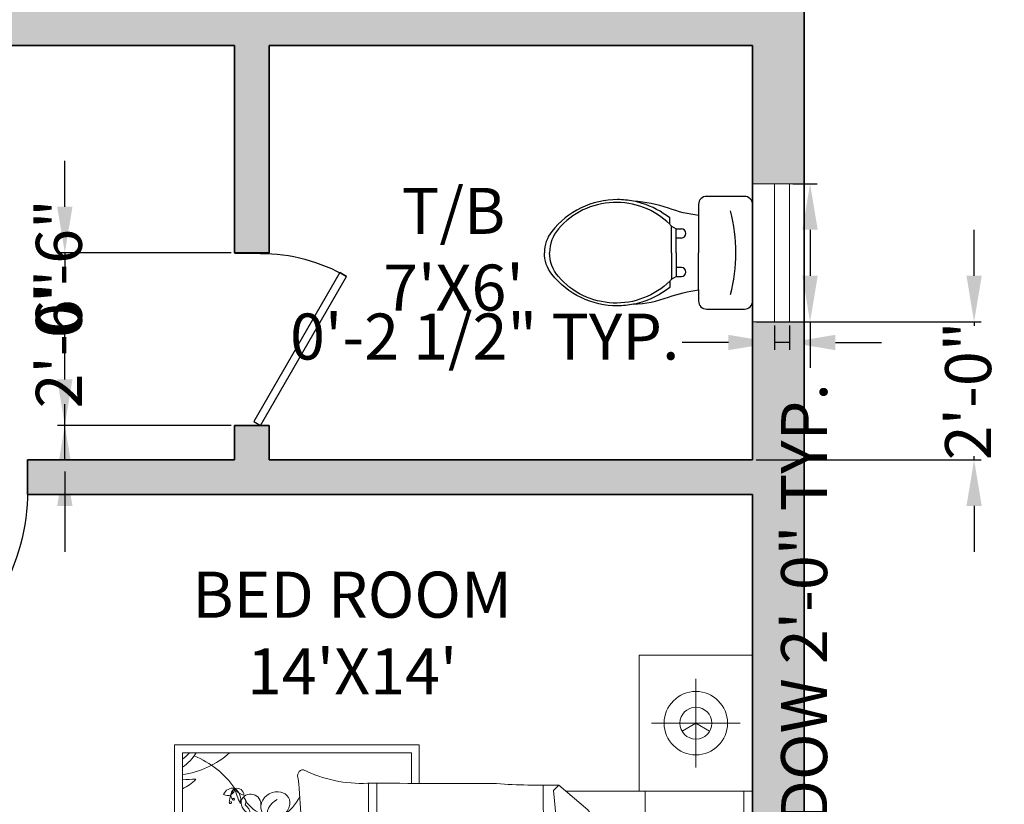
# Model space of a CAD drawing. Units: inches. Extents: x 2073 to 2646, y 2372 to 3017.
# Tile 3 of 8: x 2396 to 2567, y 2550 to 2686. Entities that reach past the tile are written whole.
import ezdxf

# ---------------------------------------------------------------- set-up
doc = ezdxf.new("R2010")
doc.units = ezdxf.units.IN
for name, color, linetype, lineweight in [('A-ANNO-DIMS', 2, 'Continuous', 18), ('A-AREA-IDEN', 7, 'Continuous', 25), ('A-DOOR', 3, 'Continuous', 25), ('A-FLOR-FIXT', 9, 'Continuous', 18), ('A-FURN', 8, 'Continuous', 18), ('A-GLAZ', 4, 'Continuous', 18), ('A-WALL', 7, 'Continuous', 35), ('A-WALL-PATT', 30, 'Continuous', 13)]:
    doc.layers.add(name, color=color, linetype=linetype, lineweight=lineweight)
doc.layers.add('WC-Detail_dwgmodels.com', color=251, linetype='Continuous')
doc.layers.add('WC-Outline_dwgmodels.com', color=250, linetype='Continuous')
doc.styles.get("Standard").update_dxf_attribs({"font": 'arial.ttf'})
doc.dimstyles.new('ISO-25', dxfattribs={"dimtxt": 8, "dimasz": 8, "dimexe": 1.25, "dimexo": 0.625, "dimtad": 0, "dimdec": 1, "dimlunit": 4, "dimtxsty": 'Standard', "dimcen": 2.5, "dimadec": 0, "dimazin": 0, "dimtfac": 1, "dimtdec": 1, "dimtmove": 0, "dimatfit": 3, "dimfxl": 1, "dimarcsym": 0})

# ---------------------------------------------------------------- blocks, each defined once
blk = doc.blocks.new('pan')
at = {"layer": 'WC-Detail_dwgmodels.com'}
for p, q in [((2373.44, 3021.91), (2373.44, 3022.64)), ((2374.73, 3022.64), (2374.73, 3021.91)), ((2378.86, 3022.64), (2378.86, 3021.91)), ((2380.15, 3021.91), (2380.15, 3022.64)), ((2373.08, 3021.25), (2373.44, 3021.91)), ((2374.73, 3021.91), (2373.44, 3021.91)), ((2376.79, 3021.91), (2374.73, 3021.91)), ((2376.79, 3021.91), (2378.86, 3021.91)), ((2378.86, 3021.91), (2380.15, 3021.91)), ((2380.51, 3021.25), (2380.15, 3021.91))]:
    blk.add_line(p, q, dxfattribs=at)
for points in [[(2373.08, 3021.25, 0.008985), (2372.8, 3020.99, 0.182634)], [(2376.79, 3021.25), (2373.08, 3021.25, 0.008985)], [(2376.79, 3021.25), (2380.51, 3021.25, -0.444938)], [(2380.51, 3021.25, -0.008985), (2380.79, 3020.99, -0.182634)], [(2372.8, 3020.99, 0.434217), (2373.44, 3005.35, 0.182634), (2376.79, 3004.12, 2.693815)], [(2371.91, 3020.99, 0.094048), (2369.85, 3017.12, 0.16845)], [(2372.8, 3020.99), (2371.91, 3020.99, 0.416606)], [(2380.79, 3020.99, -0.434217), (2380.15, 3005.35, -0.182634), (2376.79, 3004.12, -2.693815)], [(2380.79, 3020.99), (2381.68, 3020.99, -0.416606)], [(2381.68, 3020.99, -0.105447), (2383.88, 3016.61, -0.16845)], [(2369.85, 3017.12, 0.026594), (2369.55, 3015.91, 0.16845)], [(2383.88, 3016.61, -0.015301), (2384.04, 3015.91, -0.16845)]]:
    blk.add_lwpolyline(points, format="xyb", dxfattribs=at)
for centre, radius, start, end in [((2376.81, 3007.03), 23.26, 90.028, 104.6712), ((2376.78, 3007.03), 23.26, 75.3288, 89.972), ((2374.08, 3022.64), 0.645, 0, 180), ((2379.51, 3022.64), 0.645, 0, 180)]:
    blk.add_arc(centre, radius, start, end, dxfattribs=at)
at = {"layer": 'WC-Outline_dwgmodels.com'}
for points in [[(2383.59, 3025.06, 0.414214), (2384.72, 3026.19), (2384.72, 3031.5, 0.414214), (2383.59, 3032.64), (2376.79, 3032.64), (2370, 3032.64, 0.414214), (2368.87, 3031.5), (2368.87, 3026.19, 0.414214), (2370, 3025.06), (2371.56, 3025.06, -0.052345), (2370.54, 3020.81, 0.071131), (2369.55, 3015.91, 0.160777)], [(2371.56, 3025.06), (2376.79, 3025.06, 0.414214)], [(2382.03, 3025.06), (2376.79, 3025.06, -0.414214)], [(2384.04, 3015.91, 0.071131), (2383.05, 3020.81, -0.052345), (2382.03, 3025.06), (2383.59, 3025.06, 0.414214)], [(2369.55, 3015.91, 0.048023), (2369.32, 3013.67, 0.16845)], [(2384.04, 3015.91, -0.048023), (2384.27, 3013.67, -0.16845)], [(2369.32, 3013.67, 0.230343), (2373.8, 3004.42, 0.16845), (2376.79, 3003.38, 2.883082)], [(2384.27, 3013.67, -0.230343), (2379.79, 3004.42, -0.16845), (2376.79, 3003.38, -2.883082)]]:
    blk.add_lwpolyline(points, format="xyb", dxfattribs=at)
blk = doc.blocks.new('bed')
at = {"color": 0}
for p, q in [((2249.53, 3172.75), (2367.64, 3172.75)), ((2273.15, 3172.75), (2273.15, 3140.33)), ((2261.34, 3155.19), (2261.34, 3170.62)), ((2344.02, 3171.23), (2273.15, 3171.23)), ((2355.83, 3155.19), (2355.83, 3170.62)), ((2269.06, 3162.9), (2253.62, 3162.9)), ((2348.11, 3162.9), (2363.55, 3162.9)), ((2273.15, 3154.08), (2344.02, 3154.08)), ((2289.56, 3150.57), (2302.44, 3154.08)), ((2305.6, 3154.08), (2299.13, 3145.07)), ((2280.95, 3147.46), (2289.56, 3150.57)), ((2343.7, 3149.18), (2301.65, 3148.59)), ((2276.4, 3144.12), (2280.95, 3147.46)), ((2343.66, 3147.96), (2300.77, 3147.36)), ((2299.13, 3145.07), (2296.5, 3138.14)), ((2272.09, 3139.1), (2276.4, 3144.12)), ((2343.6, 3143.03), (2298.28, 3142.85)), ((2343.59, 3144.24), (2298.75, 3144.07)), ((2273.05, 3138.14), (2272.09, 3139.1)), ((2277.84, 3138.62), (2273.05, 3138.14)), ((2283.82, 3138.14), (2277.84, 3138.62)), ((2289.08, 3137.42), (2283.82, 3138.14)), ((2296.5, 3138.14), (2296.02, 3135.03)), ((2292.19, 3135.99), (2289.08, 3137.42)), ((2296.02, 3135.03), (2292.19, 3135.99)), ((2265.12, 3114.85), (2271.8, 3114.85)), ((2265.12, 3072.3), (2265.12, 3114.85)), ((2344.68, 3114.85), (2351.23, 3114.85)), ((2351.23, 3114.85), (2351.23, 3072.3)), ((2271.8, 3113.48), (2266.49, 3113.48)), ((2266.49, 3113.48), (2266.49, 3073.67)), ((2349.86, 3113.48), (2344.65, 3113.48)), ((2349.86, 3073.67), (2349.86, 3113.48)), ((2344.56, 3107.48), (2271.79, 3107.48)), ((2344.67, 3106.01), (2271.79, 3106.01)), ((2332.56, 3094.41), (2284.61, 3094.41)), ((2278.13, 3085.65), (2277.87, 3086.98)), ((2286.38, 3085.65), (2286.64, 3086.98)), ((2329.96, 3085.65), (2329.7, 3086.98)), ((2338.22, 3085.65), (2338.48, 3086.98)), ((2266.49, 3073.67), (2349.86, 3073.67)), ((2351.23, 3072.3), (2265.12, 3072.3))]:
    blk.add_line(p, q, dxfattribs=at)
for points in [[(2273.15, 3153.06), (2249.53, 3153.06), (2249.53, 3172.75)], [(2344.02, 3172.75), (2344.02, 3153.06), (2367.64, 3153.06), (2367.64, 3172.75)], [(2261.34, 3162.9), (2262.72, 3165.29)], [(2355.83, 3162.9), (2354.45, 3165.29)], [(2261.34, 3162.9), (2262.72, 3160.52)], [(2355.83, 3162.9), (2354.45, 3160.52)]]:
    blk.add_lwpolyline(points, dxfattribs=at)
for points in [[(2279.94, 3169.8, 0.074897), (2280.08, 3162.09, -0.472817)], [(2308.03, 3161.66, 0.14099), (2308.27, 3169.53, 0.235245)], [(2313.08, 3161.66, -0.14099), (2312.84, 3169.53, -0.235245)], [(2337.23, 3169.8, -0.074897), (2337.09, 3162.09, 0.472817)], [(2271.85, 3128.28, 0.001242), (2271.79, 3105.87, -0.127202), (2269.42, 3094.7)], [(2344.52, 3108.41, 0.056112), (2345.38, 3101.91, 0.095341), (2347.04, 3095.66)]]:
    blk.add_lwpolyline(points, format="xyb", dxfattribs=at)
for centre, radius in [((2261.34, 3162.9), 5.51), ((2355.83, 3162.9), 5.51), ((2261.34, 3162.9), 2.76), ((2355.83, 3162.9), 2.76), ((2284.95, 3081.37), 0.301), ((2331.4, 3081.37), 0.301), ((2282.98, 3078.2), 0.301), ((2333.36, 3078.2), 0.301)]:
    blk.add_circle(centre, radius, dxfattribs=at)
for centre, radius, start, end in [((2345.04, 4293.82), 1125.9, 266.68521, 267.14978), ((2296.12, 3127.06), 42.84, 82.2196, 99.497), ((2305.17, 3148.71), 21.05, 81.5249, 103.96), ((2314.46, 3163.91), 5.84, 63.3437, 106.1026), ((2323.22, 3149.14), 20.76, 76.3427, 101.1841), ((2272.13, 4293.82), 1125.9, 272.85022, 273.31479), ((2294.98, 3158.99), 15.22, 155.1316, 191.7583), ((2322.19, 3158.99), 15.22, 348.2417, 24.8684), ((2294.11, 3157.71), 14.47, 354.0129, 15.8293), ((2327, 3157.71), 14.47, 164.1707, 185.9871), ((2284.15, 3171.19), 15.83, 255.1039, 281.0369), ((2292.48, 3182.44), 27.45, 258.0397, 289.2615), ((2303.6, 3176.44), 20.83, 259.8617, 283.6238), ((2315.25, 3161.88), 6.26, 245.0183, 288.5407), ((2326.19, 3170.02), 15.03, 243.8761, 286.1746), ((2333.02, 3171.19), 15.83, 258.9631, 284.8961), ((2555.75, 3139.65), 212.22, 176.1, 180.9282), ((2163.8, 3136.16), 108.33, 355.8294, 1.553), ((2274.12, 3180.92), 44.58, 267.4519, 281.3392), ((2284.77, 3127.79), 9.61, 66.2616, 101.3392), ((2304.22, 3179.66), 45.8, 250.1194, 259.3383), ((2620.36, 3131.93), 276.84, 179.1145, 184.8735), ((2295.75, 3134.94), 0.285, 268.8623, 19.7536), ((2346.15, 3095.06), 1.08, 246.5219, 33.8264), ((2270.51, 3094.78), 1.09, 183.98, 297.3412), ((2283.2, 2971.46), 122.95, 89.3433, 95.6887), ((2270.05, 3086.09), 8.94, 33.6671, 63.2997), ((2282.03, 3091.41), 4.56, 145.785, 184.7304), ((2273.33, 3093.53), 4.89, 328.8218, 9.1554), ((2279.39, 3093.1), 1.42, 120.0293, 142.325), ((2277.12, 3092.26), 3.76, 289.2822, 29.1751), ((2278.79, 3093.38), 1.77, 311.5653, 23.8354), ((2279.39, 3093.1), 1.42, 44.4517, 63.558), ((2287.39, 3092.26), 3.76, 150.8249, 250.7178), ((2285.72, 3093.38), 1.77, 156.1646, 228.4347), ((2285.12, 3093.1), 1.42, 113.229, 135.5483), ((2285.12, 3093.1), 1.42, 37.675, 66.7144), ((2282.48, 3091.41), 4.56, 355.2696, 34.215), ((2291.18, 3093.53), 4.89, 169.7133, 211.1782), ((2294.46, 3086.09), 8.94, 111.4941, 146.3329), ((2321.89, 3086.09), 8.94, 33.6671, 68.5059), ((2333.87, 3091.41), 4.56, 145.785, 184.7304), ((2325.17, 3093.53), 4.89, 328.8218, 10.2867), ((2331.23, 3093.1), 1.42, 113.2856, 142.325), ((2328.96, 3092.26), 3.76, 289.2822, 29.1751), ((2331.23, 3093.1), 1.42, 44.4517, 66.7144), ((2330.63, 3093.38), 1.77, 311.5653, 23.8354), ((2336.18, 2979.53), 114.93, 85.2402, 91.8035), ((2339.23, 3092.26), 3.76, 150.8249, 250.7178), ((2337.56, 3093.38), 1.77, 156.1646, 228.4347), ((2336.96, 3093.1), 1.42, 106.6343, 135.5483), ((2336.96, 3093.1), 1.42, 37.675, 72.5814), ((2334.32, 3091.41), 4.56, 355.2696, 34.215), ((2343.02, 3093.53), 4.89, 169.249, 211.1782), ((2346.3, 3086.09), 8.94, 113.6453, 146.3329), ((2275.26, 3090.38), 1.99, 84.4856, 181.0538), ((2274.65, 3088.91), 3.55, 355.2933, 76.921), ((2281.57, 3090.25), 2.42, 131.5653, 195.1471), ((2276.55, 3091.58), 3.4, 7.436, 29.9149), ((2282.94, 3090.25), 2.42, 344.8529, 48.4347), ((2287.96, 3091.58), 3.4, 150.0851, 172.564), ((2289.86, 3088.91), 3.55, 103.079, 184.7067), ((2289.25, 3090.38), 1.99, 358.9462, 95.5144), ((2327.09, 3090.38), 1.99, 84.4856, 181.0538), ((2326.48, 3088.91), 3.55, 355.2933, 76.921), ((2333.4, 3090.25), 2.42, 131.5653, 195.1471), ((2328.39, 3091.58), 3.4, 7.436, 29.9149), ((2334.78, 3090.25), 2.42, 344.8529, 48.4347), ((2339.8, 3091.58), 3.4, 150.0851, 172.564), ((2341.7, 3088.91), 3.55, 103.079, 184.7067), ((2341.09, 3090.38), 1.99, 358.9462, 95.5144), ((2276.08, 3090.1), 2.82, 174.9449, 262.8857), ((2277.18, 3091.17), 2.74, 201.5819, 291.4221), ((2276.66, 3088.19), 2.94, 299.9085, 73.1337), ((2287.85, 3088.19), 2.94, 106.8663, 240.0915), ((2287.32, 3091.17), 2.74, 248.5779, 338.4181), ((2288.43, 3090.1), 2.82, 277.1143, 5.0551), ((2327.91, 3090.1), 2.82, 174.9449, 262.8857), ((2329.02, 3091.17), 2.74, 201.5819, 291.4221), ((2328.5, 3088.19), 2.94, 299.9085, 73.1337), ((2339.68, 3088.19), 2.94, 106.8663, 240.0915), ((2339.16, 3091.17), 2.74, 248.5779, 338.4181), ((2340.27, 3090.1), 2.82, 277.1143, 5.0551), ((2275.58, 3090.72), 3.43, 272.3591, 324.0401), ((2271.86, 3089), 6.34, 326.2883, 356.5076), ((2282.03, 3091.41), 4.56, 212.7011, 216.3445), ((2278.52, 3089.43), 0.733, 257.3041, 15.1471), ((2282.59, 3088.31), 0.228, 102.7051, 280.4384), ((2282.57, 3088.45), 0.37, 280.4384, 100.4136), ((2285.99, 3089.43), 0.733, 164.8529, 282.6959), ((2282.48, 3091.41), 4.56, 323.6555, 327.2989), ((2288.92, 3090.72), 3.43, 215.9599, 267.6409), ((2292.65, 3089), 6.34, 183.4924, 213.7117), ((2327.42, 3090.72), 3.43, 272.3591, 324.0401), ((2323.7, 3089), 6.34, 326.2883, 356.5076), ((2333.87, 3091.41), 4.56, 212.7011, 216.3445), ((2330.36, 3089.43), 0.733, 257.3041, 15.1471), ((2333.78, 3088.45), 0.37, 79.5864, 259.5616), ((2333.75, 3088.31), 0.228, 259.5616, 77.2949), ((2337.82, 3089.43), 0.733, 164.8529, 282.6959), ((2334.32, 3091.41), 4.56, 323.6555, 327.2989), ((2340.76, 3090.72), 3.43, 215.9599, 267.6409), ((2344.49, 3089), 6.34, 183.4924, 213.7117), ((2275.43, 3085.55), 1.77, 80.264, 250.8688), ((2271.91, 3089.45), 5.58, 301.2614, 341.7045), ((2290.78, 3082.37), 9.78, 153.0032, 159.8941), ((2292.6, 3089.45), 5.58, 198.2955, 238.7386), ((2289.08, 3085.55), 1.77, 289.1312, 99.736), ((2309.5, 3071.59), 15.42, 94.4623, 172.255), ((2309.57, 3085.82), 1.71, 137.7873, 219.1145), ((2307.63, 3085.87), 1.29, 298.5391, 58.3627), ((2309.53, 3086.61), 1.28, 63.0274, 163.8037), ((2308.24, 3089.6), 2.63, 271.4585, 315.3727), ((2309.31, 3084.75), 2.44, 45.5411, 114.3101), ((2311.53, 3097.27), 10.79, 252.593, 267.2582), ((2309.56, 3086.92), 1.26, 177.7585, 283.852), ((2311.99, 3088.23), 3.9, 198.9159, 238.011), ((2310.98, 3084.75), 2.44, 65.6899, 134.4589), ((2308.75, 3097.27), 10.79, 272.7418, 287.407), ((2310.75, 3086.61), 1.28, 16.1963, 116.9726), ((2312.05, 3089.6), 2.63, 224.6273, 268.5415), ((2308.29, 3088.23), 3.9, 301.989, 341.0841), ((2310.72, 3086.92), 1.26, 256.148, 2.2415), ((2312.66, 3085.87), 1.29, 121.6373, 241.4609), ((2310.71, 3085.82), 1.71, 320.8855, 42.2127), ((2310.28, 3075.15), 11.94, 352.8636, 81.8197), ((2327.26, 3085.55), 1.77, 80.264, 250.8688), ((2323.75, 3089.45), 5.58, 301.2614, 341.7045), ((2325.57, 3082.37), 9.78, 20.1059, 26.9968), ((2344.44, 3089.45), 5.58, 198.2955, 238.7386), ((2340.92, 3085.55), 1.77, 289.1312, 99.736), ((2275, 3086.08), 2.21, 265.969, 344.3045), ((2277.38, 3083.14), 2.36, 96.1662, 141.5825), ((2281.29, 3084.79), 0.62, 101.3256, 154.4621), ((2280.4, 3086.9), 1.87, 280.2588, 300.656), ((2280.83, 3088.39), 3.33, 268.3264, 277.1302), ((2290.78, 3082.37), 9.78, 163.5842, 183.8277), ((2279.99, 3086.89), 1.9, 308.2101, 316.3071), ((2281.16, 3085.65), 0.567, 278.3432, 4.2869), ((2280.84, 3086.14), 0.99, 300.656, 332.6341), ((2281.59, 3085.49), 0.241, 55.7657, 157.4417), ((2281.96, 3085.71), 0.241, 84.3784, 186.0543), ((2281.74, 3086.68), 0.99, 269.1859, 301.164), ((2282.03, 3086.17), 0.567, 237.5332, 323.4768), ((2281.48, 3087.78), 1.9, 285.5129, 293.6099), ((2282.72, 3085.65), 0.62, 87.3579, 140.4944), ((2281.28, 3087.43), 1.87, 301.164, 321.5612), ((2279.77, 3087.76), 3.33, 324.6898, 333.4936), ((2287.12, 3083.14), 2.36, 38.4175, 83.8338), ((2289.51, 3086.08), 2.21, 195.6955, 274.031), ((2309.83, 3085.86), 0.167, 283.852, 219.9245), ((2310.03, 3085.09), 0.192, 238.011, 71.5592), ((2310.06, 3085.18), 0.093, 71.5592, 188.0167), ((2310.25, 3085.09), 0.192, 108.4408, 301.989), ((2310.22, 3085.18), 0.093, 351.9833, 108.4408), ((2310.44, 3085.92), 0.101, 320.1909, 256.0209), ((2326.84, 3086.08), 2.21, 265.969, 344.3045), ((2329.22, 3083.14), 2.36, 96.1662, 141.5825), ((2335.06, 3087.43), 1.87, 218.4388, 238.836), ((2333.63, 3085.65), 0.62, 39.5056, 92.6421), ((2336.58, 3087.76), 3.33, 206.5064, 215.3102), ((2334.32, 3086.17), 0.567, 216.5232, 302.4668), ((2334.61, 3086.68), 0.99, 238.836, 270.8141), ((2334.87, 3087.78), 1.9, 246.3901, 254.4871), ((2334.38, 3085.71), 0.241, 353.9457, 95.6216), ((2334.76, 3085.49), 0.241, 22.5583, 124.2343), ((2335.19, 3085.65), 0.567, 175.7131, 261.6568), ((2335.5, 3086.14), 0.99, 207.3659, 239.344), ((2325.57, 3082.37), 9.78, 356.1723, 16.4158), ((2336.35, 3086.89), 1.9, 223.6929, 231.7899), ((2335.95, 3086.9), 1.87, 239.344, 259.7412), ((2335.52, 3088.39), 3.33, 262.8698, 271.6736), ((2335.06, 3084.79), 0.62, 25.5379, 78.6744), ((2341.35, 3086.08), 2.21, 195.6955, 274.031), ((2338.96, 3083.14), 2.36, 38.4175, 83.8338), ((2273.92, 3083.1), 1.28, 92.9516, 193.728), ((2271.31, 3085.04), 2.63, 301.3827, 345.2969), ((2274.66, 3081.37), 2.44, 75.4653, 144.2343), ((2270.34, 3093.33), 10.79, 282.5173, 297.1824), ((2275.06, 3083.63), 1.09, 63.9755, 143.2681), ((2279.54, 3083.62), 0.502, 101.5637, 142.6358), ((2279.12, 3083.15), 0.301, 273.2768, 86.7232), ((2279.47, 3083.44), 0.287, 91.1081, 181.8675), ((2279.78, 3082.86), 0.622, 80.3487, 133.6538), ((2279.13, 3084.01), 0.723, 288.7263, 352.5032), ((2279.66, 3082.21), 0.985, 83.0852, 105.7171), ((2279.63, 3083.98), 0.232, 345.2356, 144.9248), ((2279.84, 3083.22), 0.259, 317.6792, 80.3487), ((2289.45, 3083.63), 1.09, 36.7319, 116.0245), ((2289.85, 3081.37), 2.44, 35.7657, 104.5347), ((2294.17, 3093.33), 10.79, 242.8176, 257.4827), ((2290.59, 3083.1), 1.28, 346.272, 87.0484), ((2293.2, 3085.04), 2.63, 194.7031, 238.6173), ((2325.76, 3083.1), 1.28, 92.9516, 193.728), ((2323.15, 3085.04), 2.63, 301.3827, 345.2969), ((2326.5, 3081.37), 2.44, 75.4653, 144.2343), ((2322.18, 3093.33), 10.79, 282.5173, 297.1824), ((2326.9, 3083.63), 1.09, 63.9755, 143.2681), ((2336.51, 3083.22), 0.259, 99.6513, 222.3208), ((2336.57, 3082.86), 0.622, 46.3462, 99.6513), ((2336.72, 3083.98), 0.232, 35.0752, 194.7644), ((2337.21, 3084.01), 0.723, 187.4968, 251.2737), ((2336.69, 3082.21), 0.985, 74.2829, 96.9148), ((2336.88, 3083.44), 0.287, 358.1325, 88.8919), ((2336.81, 3083.62), 0.502, 37.3642, 78.4363), ((2337.23, 3083.15), 0.301, 93.2768, 266.7232), ((2341.29, 3083.63), 1.09, 36.7319, 116.0245), ((2341.69, 3081.37), 2.44, 35.7657, 104.5347), ((2346, 3093.33), 10.79, 242.8176, 257.4827), ((2345.04, 3085.04), 2.63, 194.7031, 238.6173), ((2342.42, 3083.1), 1.28, 346.272, 87.0484), ((2255.01, 3071.59), 15.42, 7.745, 41.8856), ((2281.39, 3070.07), 15.42, 124.3865, 158.5908), ((2274.35, 3082.43), 1.71, 167.7115, 249.0387), ((2272.64, 3081.51), 1.29, 328.4633, 88.2869), ((2275.25, 3085.73), 3.9, 228.8402, 267.9352), ((2273.8, 3083.38), 1.26, 207.6827, 313.7762), ((2274.56, 3082.59), 0.167, 313.7762, 249.7183), ((2275.1, 3082.12), 0.093, 101.4834, 217.9409), ((2275.12, 3082.03), 0.192, 267.9352, 101.4834), ((2279.53, 3082.6), 0.497, 217.7621, 259.0403), ((2280.07, 3083.26), 0.913, 203.4276, 227.6104), ((2279.66, 3083.37), 0.492, 229.7889, 317.6792), ((2279.11, 3082.33), 0.699, 355.053, 68.3618), ((2279.58, 3082.29), 0.231, 232.4737, 355.053), ((2272.84, 3074.04), 11.21, 43.1541, 52.0459), ((2280.59, 3080.82), 0.62, 101.3256, 154.4621), ((2279.29, 3082.92), 1.9, 308.2101, 316.3071), ((2280.45, 3081.67), 0.567, 278.3432, 4.2869), ((2280.14, 3082.17), 0.99, 300.656, 332.6341), ((2280.88, 3081.52), 0.241, 55.7657, 157.4417), ((2285.91, 3082.12), 4.9, 184.756, 209.2041), ((2292.97, 3092.56), 16.14, 222.2412, 232.1744), ((2283.38, 3081.51), 0.833, 272.8499, 356.1226), ((2282.65, 3081.81), 1.37, 304.5369, 16.3699), ((2284.55, 3081.43), 0.97, 127.3105, 187.9252), ((2283.22, 3081.54), 0.996, 355.0106, 41.658), ((2284.62, 3081.78), 0.41, 126.1046, 271.4281), ((2284.57, 3081.9), 0.295, 353.7526, 131.7054), ((2284.3, 3081.55), 0.414, 0.0645, 61.1507), ((2284.39, 3081.9), 0.473, 311.8413, 355.7877), ((2285.37, 3081.83), 0.502, 101.5637, 176.365), ((2285.3, 3081.65), 0.287, 91.1081, 181.8675), ((2285.61, 3081.07), 0.622, 80.3487, 133.6538), ((2284.96, 3082.22), 0.723, 288.7263, 352.5032), ((2285.49, 3080.43), 0.985, 83.0852, 105.7171), ((2285.46, 3082.19), 0.232, 345.2356, 144.9248), ((2285.67, 3081.43), 0.259, 317.6792, 80.3487), ((2286.41, 3075.61), 5.88, 87.1071, 94.7585), ((2289.39, 3082.03), 0.192, 78.5166, 272.0648), ((2289.26, 3085.73), 3.9, 272.0648, 311.1598), ((2289.41, 3082.12), 0.093, 322.0591, 78.5166), ((2290.71, 3083.38), 1.26, 226.2238, 332.3173), ((2289.97, 3082.66), 0.101, 290.2667, 226.2271), ((2291.87, 3081.51), 1.29, 91.7131, 211.5367), ((2290.16, 3082.43), 1.71, 290.9613, 12.2885), ((2283.12, 3070.07), 15.42, 21.4092, 55.6135), ((2333.23, 3070.07), 15.42, 124.3865, 158.5908), ((2326.19, 3082.43), 1.71, 167.7115, 249.0387), ((2325.64, 3083.38), 1.26, 207.6827, 313.7762), ((2327.09, 3085.73), 3.9, 228.8402, 267.9352), ((2324.48, 3081.51), 1.29, 328.4633, 88.2869), ((2326.39, 3082.59), 0.167, 313.7762, 249.7183), ((2326.93, 3082.12), 0.093, 101.4834, 217.9409), ((2326.95, 3082.03), 0.192, 267.9352, 101.4834), ((2329.94, 3075.61), 5.88, 85.2415, 92.8929), ((2330.68, 3081.43), 0.259, 99.6513, 222.3208), ((2330.74, 3081.07), 0.622, 46.3462, 99.6513), ((2330.89, 3082.19), 0.232, 35.0752, 194.7644), ((2331.38, 3082.22), 0.723, 187.4968, 251.2737), ((2330.86, 3080.43), 0.985, 74.2829, 96.9148), ((2331.05, 3081.65), 0.287, 358.1325, 88.8919), ((2330.98, 3081.83), 0.502, 3.635, 78.4363), ((2331.77, 3081.9), 0.295, 48.2946, 186.2474), ((2331.95, 3081.9), 0.473, 184.2123, 228.1587), ((2332.05, 3081.55), 0.414, 118.8493, 179.9355), ((2331.73, 3081.78), 0.41, 268.5719, 53.8954), ((2333.13, 3081.54), 0.996, 138.342, 184.9894), ((2332.97, 3081.51), 0.833, 183.8774, 267.1501), ((2333.7, 3081.81), 1.37, 163.6301, 235.4631), ((2331.79, 3081.43), 0.97, 352.0748, 52.6895), ((2323.38, 3092.56), 16.14, 307.8256, 317.7588), ((2330.44, 3082.12), 4.9, 330.7959, 355.244), ((2343.51, 3074.04), 11.21, 127.9541, 136.8459), ((2335.46, 3081.52), 0.241, 22.5583, 124.2343), ((2335.89, 3081.67), 0.567, 175.7131, 261.6568), ((2336.21, 3082.17), 0.99, 207.3659, 239.344), ((2337.06, 3082.92), 1.9, 223.6929, 231.7899), ((2335.76, 3080.82), 0.62, 25.5379, 78.6744), ((2336.68, 3083.37), 0.492, 222.3208, 310.2111), ((2337.24, 3082.33), 0.699, 111.6382, 184.947), ((2336.77, 3082.29), 0.231, 184.947, 307.5263), ((2336.28, 3083.26), 0.913, 312.3896, 336.5724), ((2336.82, 3082.6), 0.497, 280.9597, 322.2379), ((2341.23, 3082.03), 0.192, 78.5166, 272.0648), ((2341.1, 3085.73), 3.9, 272.0648, 311.1598), ((2341.25, 3082.12), 0.093, 322.0591, 78.5166), ((2342.55, 3083.38), 1.26, 226.2238, 332.3173), ((2341.81, 3082.66), 0.101, 290.2667, 226.2271), ((2343.7, 3081.51), 1.29, 91.7131, 211.5367), ((2341.99, 3082.43), 1.71, 290.9613, 12.2885), ((2334.95, 3070.07), 15.42, 21.4092, 55.6135), ((2361.34, 3071.59), 15.42, 138.1144, 172.255), ((2279.69, 3082.92), 1.87, 280.2588, 300.656), ((2280.12, 3084.42), 3.33, 268.3264, 277.1302), ((2280.79, 3079.73), 0.336, 146.8636, 236.9021), ((2285.53, 3087.13), 8.79, 235.1882, 238.8844), ((2281.37, 3080.22), 0.909, 199.4799, 267.6828), ((2281.59, 3079.47), 0.262, 311.8703, 134.2646), ((2282.36, 3080.66), 1.37, 247.2305, 319.0635), ((2286.41, 3075.61), 5.88, 120.544, 139.818), ((2283.06, 3078.85), 0.97, 70.0041, 130.6188), ((2282.43, 3080.03), 0.996, 297.7043, 344.3516), ((2282.79, 3081.18), 0.807, 321.7607, 7.9252), ((2282.96, 3080.02), 0.807, 8.7227, 54.8872), ((2283, 3079.38), 1.37, 0.278, 72.111), ((2283.62, 3079.88), 0.833, 20.5253, 88.5375), ((2284.72, 3080.29), 0.97, 188.7227, 249.3375), ((2284.32, 3080.8), 0.298, 148.0499, 225.6268), ((2286.41, 3075.61), 5.88, 113.0501, 113.8477), ((2284.87, 3080.46), 0.948, 104.7558, 148.0499), ((2284.34, 3081.14), 0.594, 247.4086, 351.4386), ((2283.47, 3079.81), 0.996, 334.9899, 21.6373), ((2284.51, 3081.11), 0.199, 262.906, 7.132), ((2285.36, 3080.81), 0.497, 151.2196, 259.0403), ((2285.9, 3081.47), 0.913, 203.4276, 227.6104), ((2285.5, 3081.59), 0.492, 229.7889, 317.6792), ((2284.94, 3080.54), 0.699, 355.053, 68.3618), ((2285.41, 3080.5), 0.231, 232.4737, 355.053), ((2330.85, 3081.59), 0.492, 222.3208, 310.2111), ((2331.41, 3080.54), 0.699, 111.6382, 184.947), ((2330.94, 3080.5), 0.231, 184.947, 307.5263), ((2330.45, 3081.47), 0.913, 312.3896, 336.5724), ((2330.99, 3080.81), 0.497, 280.9597, 28.7804), ((2332.01, 3081.14), 0.594, 188.5614, 292.5914), ((2331.84, 3081.11), 0.199, 172.868, 277.094), ((2331.48, 3080.46), 0.948, 31.9501, 75.2442), ((2332.87, 3079.81), 0.996, 158.3627, 205.0101), ((2332.73, 3079.88), 0.833, 91.4625, 159.4747), ((2333.34, 3079.38), 1.37, 107.889, 179.722), ((2331.63, 3080.29), 0.97, 290.6625, 351.2773), ((2329.94, 3075.61), 5.88, 66.1523, 66.9499), ((2332.03, 3080.8), 0.298, 314.3732, 31.9501), ((2333.39, 3080.02), 0.807, 125.1128, 171.2773), ((2333.55, 3081.18), 0.807, 172.0748, 218.2393), ((2329.94, 3075.61), 5.88, 40.182, 59.456), ((2333.29, 3078.85), 0.97, 49.3812, 109.9959), ((2333.99, 3080.66), 1.37, 220.9365, 292.7695), ((2333.91, 3080.03), 0.996, 195.6484, 242.2957), ((2334.75, 3079.47), 0.262, 45.7354, 228.1297), ((2334.98, 3080.22), 0.909, 272.3172, 340.5201), ((2330.82, 3087.13), 8.79, 301.1156, 304.8118), ((2336.65, 3082.92), 1.87, 239.344, 259.7412), ((2335.55, 3079.73), 0.336, 303.0979, 33.1364), ((2336.22, 3084.42), 3.33, 262.8698, 271.6736), ((2281.27, 3079.88), 0.783, 212.8155, 277.3992), ((2280.81, 3079.35), 0.909, 266.9701, 338.2913), ((2276.02, 3085.84), 8.79, 302.6784, 306.3746), ((2281.04, 3078.63), 0.336, 214.3538, 304.3923), ((2281.17, 3079.91), 0.348, 238.8844, 314.2646), ((2281.09, 3079.13), 0.783, 280.3057, 17.1958), ((2281.03, 3079.05), 0.348, 306.3746, 21.7548), ((2281.59, 3079.27), 0.262, 19.3605, 201.7548), ((2286.53, 3077.08), 5.24, 153.7819, 158.2913), ((2281.9, 3080.2), 0.807, 264.4544, 310.6188), ((2285.91, 3082.12), 4.9, 214.0033, 222.4917), ((2282.49, 3079.88), 0.833, 218.3208, 298.8162), ((2282.9, 3077.29), 0.948, 104.7558, 148.0499), ((2282.65, 3078.61), 0.41, 126.1046, 271.4281), ((2282.61, 3078.72), 0.295, 353.7526, 131.7054), ((2282.33, 3078.37), 0.414, 0.0645, 61.1507), ((2282.43, 3078.73), 0.473, 311.8413, 355.7877), ((2283.4, 3078.66), 0.502, 101.5637, 176.365), ((2283.33, 3078.48), 0.287, 91.1081, 181.8675), ((2283.64, 3077.9), 0.622, 80.3487, 133.6538), ((2283.53, 3078.42), 0.492, 229.7889, 317.6792), ((2283, 3079.05), 0.723, 288.7263, 352.5032), ((2282.97, 3077.37), 0.699, 355.053, 68.3618), ((2283.52, 3077.26), 0.985, 83.0852, 105.7171), ((2283.49, 3079.02), 0.232, 345.2356, 144.9248), ((2283.7, 3078.26), 0.259, 317.6792, 80.3487), ((2308.32, 3063.33), 15.42, 94.4623, 117.4146), ((2308.39, 3077.56), 1.71, 137.7873, 219.1145), ((2306.45, 3077.61), 1.29, 298.5391, 58.3627), ((2308.35, 3078.35), 1.28, 63.0274, 163.8037), ((2307.06, 3081.34), 2.63, 271.4585, 315.3727), ((2308.13, 3076.49), 2.44, 45.5411, 114.3101), ((2310.81, 3079.97), 3.9, 198.9159, 238.011), ((2310.35, 3089), 10.79, 252.593, 267.2582), ((2308.38, 3078.66), 1.26, 177.7585, 283.852), ((2312.16, 3076.49), 2.44, 65.6899, 134.4589), ((2309.93, 3089), 10.79, 272.7418, 287.407), ((2311.93, 3078.35), 1.28, 16.1963, 116.9726), ((2313.23, 3081.34), 2.63, 224.6273, 268.5415), ((2309.47, 3079.97), 3.9, 301.989, 341.0841), ((2311.9, 3078.66), 1.26, 256.148, 2.2415), ((2313.84, 3077.61), 1.29, 121.6373, 241.4609), ((2311.89, 3077.56), 1.71, 320.8855, 42.2127), ((2311.96, 3063.33), 15.42, 62.5854, 85.5377), ((2332.65, 3078.26), 0.259, 99.6513, 222.3208), ((2332.82, 3078.42), 0.492, 222.3208, 310.2111), ((2332.71, 3077.9), 0.622, 46.3462, 99.6513), ((2332.86, 3079.02), 0.232, 35.0752, 194.7644), ((2333.35, 3079.05), 0.723, 187.4968, 251.2737), ((2333.37, 3077.37), 0.699, 111.6382, 184.947), ((2332.83, 3077.26), 0.985, 74.2829, 96.9148), ((2333.01, 3078.48), 0.287, 358.1325, 88.8919), ((2332.95, 3078.66), 0.502, 3.635, 78.4363), ((2333.85, 3079.88), 0.833, 241.1838, 321.6792), ((2333.74, 3078.72), 0.295, 48.2946, 186.2474), ((2333.92, 3078.73), 0.473, 184.2123, 228.1587), ((2334.02, 3078.37), 0.414, 118.8493, 179.9355), ((2333.7, 3078.61), 0.41, 268.5719, 53.8954), ((2333.44, 3077.29), 0.948, 31.9501, 75.2442), ((2334.44, 3080.2), 0.807, 229.3812, 275.5456), ((2330.44, 3082.12), 4.9, 317.5083, 325.9967), ((2335.25, 3079.13), 0.783, 162.8042, 259.6943), ((2334.75, 3079.27), 0.262, 338.2452, 160.6395), ((2329.82, 3077.08), 5.24, 21.7087, 26.2181), ((2335.53, 3079.35), 0.909, 201.7087, 273.0299), ((2335.18, 3079.91), 0.348, 225.7354, 301.1156), ((2335.32, 3079.05), 0.348, 158.2452, 233.6254), ((2335.08, 3079.88), 0.783, 262.6008, 327.1845), ((2340.32, 3085.84), 8.79, 233.6254, 237.3216), ((2335.3, 3078.63), 0.336, 235.6077, 325.6462), ((2282.35, 3077.63), 0.298, 148.0499, 225.6268), ((2282.37, 3077.97), 0.594, 247.4086, 351.4386), ((2282.54, 3077.94), 0.199, 262.906, 7.132), ((2283.39, 3077.64), 0.497, 151.2196, 259.0403), ((2283.93, 3078.3), 0.913, 203.4276, 227.6104), ((2283.44, 3077.33), 0.231, 232.4737, 355.053), ((2301.77, 3069.53), 7.52, 91.272, 146.5383), ((2304.47, 3068.13), 9.37, 107.8504, 143.6964), ((2309.39, 3065.49), 13.93, 124.0123, 144.053), ((2308.65, 3077.6), 0.167, 283.852, 219.9245), ((2308.85, 3076.83), 0.192, 238.011, 71.5592), ((2308.88, 3076.92), 0.093, 71.5592, 188.0167), ((2311.44, 3076.83), 0.192, 108.4408, 301.989), ((2311.4, 3076.92), 0.093, 351.9833, 108.4408), ((2311.62, 3077.66), 0.101, 320.1909, 256.0209), ((2311.82, 3076.24), 6.91, 338.117, 6.6195), ((2318.16, 3074.32), 2.77, 346.3898, 79.0739), ((2316.08, 3074.7), 3.5, 342.8609, 41.9049), ((2332.91, 3077.33), 0.231, 184.947, 307.5263), ((2332.42, 3078.3), 0.913, 312.3896, 336.5724), ((2332.95, 3077.64), 0.497, 280.9597, 28.7804), ((2333.98, 3077.97), 0.594, 188.5614, 292.5914), ((2333.81, 3077.94), 0.199, 172.868, 277.094), ((2334, 3077.63), 0.298, 314.3732, 31.9501), ((2262.74, 3069.53), 7.52, 33.4617, 60.1116), ((2260.04, 3068.13), 9.37, 36.3036, 46.4814), ((2266.95, 3071.27), 6.27, 22.5547, 48.9546), ((2249.77, 3074.64), 21.34, 357.4081, 3.6519), ((2297.56, 3071.27), 6.27, 131.0454, 157.4453), ((2314.73, 3074.64), 21.34, 176.3481, 182.5919), ((2301.61, 3074.64), 21.34, 357.4081, 3.6519), ((2318.79, 3071.27), 6.27, 22.5547, 48.9546), ((2349.39, 3071.27), 6.27, 131.0454, 157.4453), ((2366.57, 3074.64), 21.34, 176.3481, 182.5919), ((2353.6, 3069.53), 7.52, 119.8884, 146.5383), ((2356.31, 3068.13), 9.37, 133.5186, 143.6964), ((2304.01, 3065.56), 8.48, 73.5431, 107.0202), ((2307.37, 3061.19), 12.54, 94.3787, 95.6357), ((2313.97, 3052.6), 22.41, 109.7217, 109.9028), ((2316.27, 3065.56), 8.48, 72.9798, 106.4569), ((2312.91, 3061.19), 12.54, 84.3643, 85.6213), ((2306.31, 3052.6), 22.41, 70.0972, 70.2783)]:
    blk.add_arc(centre, radius, start, end, dxfattribs=at)
blk = doc.blocks.new('*U19')
for p, q in [((0, 0), (0, -6)), ((40, 0), (40, -6))]:
    blk.add_line(p, q)
blk.add_lwpolyline([(0, 0), (34.64, 20), (35.52, 18.48), (0.87, -1.52)], close=True)
blk.add_arc((0, 0), 40, 0, 30)
blk = doc.blocks.new('GLAZ-24IN')
for p, q in [((0, 24), (0, 0)), ((2.6, 24), (2.6, 0))]:
    blk.add_line(p, q)
blk = doc.blocks.new('*D27')
at = {"layer": 'A-ANNO-DIMS', "color": 0, "lineweight": -2, "transparency": 16777216}
for p, q in [((2530.32, 2657.66), (2534.54, 2657.66)), ((2533.29, 2649.66), (2533.29, 2641.66)), ((2530.32, 2633.66), (2534.54, 2633.66)), ((2533.29, 2633.66), (2533.29, 2625.66))]:
    blk.add_line(p, q, dxfattribs=at)
at = {"layer": 'A-ANNO-DIMS', "color": 0, "transparency": 16777216}
for points in [[(2531.96, 2649.66), (2534.62, 2649.66), (2533.29, 2657.66)], [(2531.96, 2641.66), (2534.62, 2641.66), (2533.29, 2633.66)]]:
    blk.add_solid(points, dxfattribs=at)
at = {"layer": 'Defpoints', "color": 0, "transparency": 16777216}
for p in [(2529.69, 2657.66), (2529.69, 2633.66), (2533.29, 2633.66)]:
    blk.add_point(p, dxfattribs=at)
at = {"layer": 'A-ANNO-DIMS', "color": 0, "transparency": 16777216, "insert": (2533.29, 2574.42), "char_height": 8, "attachment_point": 5, "rotation": 90}
blk.add_mtext('WINDOW 2\'-0" TYP.', dxfattribs=at)
blk = doc.blocks.new('*D28')
at = {"layer": 'A-ANNO-DIMS', "color": 0, "lineweight": -2, "transparency": 16777216}
for p, q in [((2527.09, 2633.04), (2527.09, 2628.81)), ((2529.69, 2633.04), (2529.69, 2628.81)), ((2519.09, 2630.06), (2511.09, 2630.06)), ((2529.69, 2630.06), (2527.09, 2630.06)), ((2537.69, 2630.06), (2545.69, 2630.06))]:
    blk.add_line(p, q, dxfattribs=at)
at = {"layer": 'A-ANNO-DIMS', "color": 0, "transparency": 16777216}
for points in [[(2519.09, 2631.4), (2519.09, 2628.73), (2527.09, 2630.06)], [(2537.69, 2631.4), (2537.69, 2628.73), (2529.69, 2630.06)]]:
    blk.add_solid(points, dxfattribs=at)
at = {"layer": 'Defpoints', "color": 0, "transparency": 16777216}
for p in [(2527.09, 2633.66), (2529.69, 2633.66), (2527.09, 2630.06)]:
    blk.add_point(p, dxfattribs=at)
at = {"layer": 'A-ANNO-DIMS', "color": 0, "transparency": 16777216, "insert": (2476.76, 2630.06), "char_height": 8, "attachment_point": 5}
blk.add_mtext('0\'-2 1/2" TYP.', dxfattribs=at)
blk = doc.blocks.new('*D29')
at = {"layer": 'A-ANNO-DIMS', "color": 0, "lineweight": -2, "transparency": 16777216}
for p, q in [((2372.17, 2524.43), (2372.17, 2532.43)), ((2366.13, 2524.43), (2373.42, 2524.43)), ((2372.17, 2487.96), (2372.17, 2516.43)), ((2366.13, 2479.96), (2373.42, 2479.96))]:
    blk.add_line(p, q, dxfattribs=at)
at = {"layer": 'A-ANNO-DIMS', "color": 0, "transparency": 16777216}
for points in [[(2370.84, 2516.43), (2373.51, 2516.43), (2372.17, 2524.43)], [(2370.84, 2487.96), (2373.51, 2487.96), (2372.17, 2479.96)]]:
    blk.add_solid(points, dxfattribs=at)
at = {"layer": 'Defpoints', "color": 0, "transparency": 16777216}
for p in [(2365.5, 2524.43), (2372.17, 2524.43), (2365.5, 2479.96)]:
    blk.add_point(p, dxfattribs=at)
at = {"layer": 'A-ANNO-DIMS', "color": 0, "transparency": 16777216, "insert": (2372.17, 2595.59), "char_height": 8, "attachment_point": 5, "rotation": 90}
blk.add_mtext('CONSOLE 3\'-8 1/2" TYP.', dxfattribs=at)
blk = doc.blocks.new('*D51')
at = {"layer": 'A-ANNO-DIMS', "color": 0, "lineweight": -2, "transparency": 16777216}
for p, q in [((2403.79, 2653.66), (2403.79, 2661.66)), ((2432.67, 2645.66), (2402.54, 2645.66)), ((2403.79, 2645.66), (2403.79, 2641.99)), ((2403.79, 2615.66), (2403.79, 2619.34)), ((2432.67, 2615.66), (2402.54, 2615.66)), ((2403.79, 2607.66), (2403.79, 2599.66))]:
    blk.add_line(p, q, dxfattribs=at)
at = {"layer": 'A-ANNO-DIMS', "color": 0, "transparency": 16777216}
for points in [[(2402.46, 2653.66), (2405.12, 2653.66), (2403.79, 2645.66)], [(2402.46, 2607.66), (2405.12, 2607.66), (2403.79, 2615.66)]]:
    blk.add_solid(points, dxfattribs=at)
at = {"layer": 'Defpoints', "color": 0, "transparency": 16777216}
for p in [(2403.79, 2645.66), (2433.29, 2645.66), (2433.29, 2615.66)]:
    blk.add_point(p, dxfattribs=at)
at = {"layer": 'A-ANNO-DIMS', "color": 0, "transparency": 16777216, "insert": (2403.79, 2630.66), "char_height": 8, "attachment_point": 5, "rotation": 90}
blk.add_mtext('2\'-6"', dxfattribs=at)
blk = doc.blocks.new('*D57')
at = {"layer": 'A-ANNO-DIMS', "color": 0, "lineweight": -2, "transparency": 16777216}
for p, q in [((2561.79, 2641.66), (2561.79, 2649.66)), ((2523.92, 2633.66), (2563.04, 2633.66)), ((2561.79, 2633.66), (2561.79, 2632.99)), ((2523.92, 2609.66), (2563.04, 2609.66)), ((2561.79, 2609.66), (2561.79, 2610.34)), ((2561.79, 2601.66), (2561.79, 2593.66))]:
    blk.add_line(p, q, dxfattribs=at)
at = {"layer": 'A-ANNO-DIMS', "color": 0, "transparency": 16777216}
for points in [[(2560.46, 2641.66), (2563.12, 2641.66), (2561.79, 2633.66)], [(2560.46, 2601.66), (2563.12, 2601.66), (2561.79, 2609.66)]]:
    blk.add_solid(points, dxfattribs=at)
at = {"layer": 'Defpoints', "color": 0, "transparency": 16777216}
for p in [(2523.29, 2633.66), (2561.79, 2633.66), (2523.29, 2609.66)]:
    blk.add_point(p, dxfattribs=at)
at = {"layer": 'A-ANNO-DIMS', "color": 0, "transparency": 16777216, "insert": (2561.79, 2621.66), "char_height": 8, "attachment_point": 5, "rotation": 90}
blk.add_mtext('2\'-0"', dxfattribs=at)
blk = doc.blocks.new('*D71')
at = {"layer": 'A-ANNO-DIMS', "color": 0, "lineweight": -2, "transparency": 16777216}
for p, q in [((2403.79, 2623.66), (2403.79, 2631.66)), ((2432.67, 2615.66), (2402.54, 2615.66)), ((2403.79, 2609.66), (2403.79, 2615.66)), ((2432.67, 2609.66), (2402.54, 2609.66)), ((2403.79, 2601.66), (2403.79, 2593.66))]:
    blk.add_line(p, q, dxfattribs=at)
at = {"layer": 'A-ANNO-DIMS', "color": 0, "transparency": 16777216}
for points in [[(2402.46, 2623.66), (2405.12, 2623.66), (2403.79, 2615.66)], [(2402.46, 2601.66), (2405.12, 2601.66), (2403.79, 2609.66)]]:
    blk.add_solid(points, dxfattribs=at)
at = {"layer": 'Defpoints', "color": 0, "transparency": 16777216}
for p in [(2403.79, 2615.66), (2433.29, 2615.66), (2433.29, 2609.66)]:
    blk.add_point(p, dxfattribs=at)
at = {"layer": 'A-ANNO-DIMS', "color": 0, "transparency": 16777216, "insert": (2403.79, 2642.92), "char_height": 8, "attachment_point": 5, "rotation": 90}
blk.add_mtext('0\'-6"', dxfattribs=at)

msp = doc.modelspace()

# ---------------------------------------------------------------- hatches: boundary and pattern name
at = {"layer": 'A-WALL-PATT'}
h = msp.add_hatch(color=256, dxfattribs=at)
h.dxf.hatch_style = 1
h.paths.add_polyline_path([(2340.29, 2948.66), (2148.29, 2948.66), (2148.29, 2924.66), (2157.29, 2924.66), (2157.29, 2939.66), (2313.29, 2939.66), (2313.29, 2885.66), (2307.29, 2885.66), (2307.29, 2879.66), (2313.29, 2879.66), (2313.29, 2777.66), (2319.29, 2777.66), (2319.29, 2831.66), (2385.29, 2831.66), (2385.29, 2825.68), (2390.69, 2825.68, -0.004149), (2391.29, 2825.68), (2391.29, 2843.66), (2385.29, 2843.66), (2385.29, 2837.66), (2319.29, 2837.66), (2319.29, 2939.66), (2340.29, 2939.66)])
h.paths.add_polyline_path([(2271.29, 2885.66), (2157.29, 2885.66), (2157.29, 2900.66), (2148.29, 2900.66), (2148.29, 2856.74), (2157.29, 2856.74), (2157.29, 2879.66), (2271.29, 2879.66)], flags=17)
h.paths.add_polyline_path([(2157.29, 2796.74), (2148.29, 2796.74), (2148.29, 2764.25), (2157.29, 2764.25)])
h.paths.add_polyline_path([(2157.29, 2681.66), (2283.29, 2681.66), (2283.29, 2687.66), (2157.29, 2687.66), (2157.29, 2704.25), (2148.29, 2704.25), (2148.29, 2621.66), (2157.29, 2621.66)])
h.paths.add_polyline_path([(2196.29, 2501.66), (2157.29, 2501.66), (2157.29, 2561.66), (2148.29, 2561.66), (2148.29, 2492.66), (2196.29, 2492.66)])
h.paths.add_polyline_path([(2295.23, 2495.54), (2295.23, 2501.66), (2256.29, 2501.66), (2256.29, 2492.66), (2295.23, 2492.66)])
h.paths.add_polyline_path([(2355.29, 2603.66), (2361.29, 2603.66), (2361.29, 2609.66), (2355.29, 2609.66), (2355.29, 2639.66), (2349.29, 2639.66), (2349.29, 2501.66), (2343.29, 2501.66), (2343.29, 2492.66), (2349.29, 2492.66), (2349.29, 2420.66), (2532.29, 2420.66), (2532.29, 2486.66), (2523.29, 2486.66), (2523.29, 2429.66), (2355.29, 2429.66)])
h.paths.add_polyline_path([(2532.29, 2633.66), (2523.29, 2633.66), (2523.29, 2609.66), (2439.29, 2609.66), (2439.29, 2615.66), (2433.29, 2615.66), (2433.29, 2609.66), (2397.31, 2609.66), (2397.31, 2604.26, -0.004149), (2397.3, 2603.66), (2523.29, 2603.66), (2523.29, 2546.66), (2532.29, 2546.66)], flags=17)
h.paths.add_polyline_path([(2532.29, 2702.66), (2523.29, 2702.66), (2523.29, 2687.66), (2385.29, 2687.66), (2343.29, 2687.66), (2343.29, 2681.66), (2349.29, 2681.66), (2349.29, 2675.66), (2355.29, 2675.66), (2355.29, 2681.66), (2433.29, 2681.66), (2433.29, 2645.66), (2439.29, 2645.66), (2439.29, 2681.66), (2523.29, 2681.66), (2523.29, 2657.66), (2532.29, 2657.66)])
h.paths.add_polyline_path([(2532.29, 2831.66), (2523.29, 2831.66), (2523.29, 2783.66), (2391.29, 2783.66), (2391.29, 2789.66), (2385.29, 2789.66), (2385.29, 2777.66), (2523.29, 2777.66), (2523.29, 2762.66), (2532.29, 2762.66)])
h.paths.add_polyline_path([(2532.29, 2948.66), (2364.29, 2948.66), (2364.29, 2939.66), (2385.29, 2939.66), (2385.29, 2873.66), (2391.29, 2873.66), (2391.29, 2939.66), (2523.29, 2939.66), (2523.29, 2891.66), (2532.29, 2891.66)])

# ---------------------------------------------------------------- linework, layer by layer
at = {"layer": 'A-GLAZ'}
for p, q in [((2523.29, 2657.66), (2532.29, 2657.66)), ((2523.29, 2633.66), (2532.29, 2633.66))]:
    msp.add_line(p, q, dxfattribs=at)
at = {"layer": 'A-WALL'}
for p, q in [((2532.29, 2420.66), (2532.29, 2948.66)), ((2355.29, 2681.66), (2433.29, 2681.66)), ((2433.29, 2645.66), (2433.29, 2681.66)), ((2439.29, 2681.66), (2523.29, 2681.66)), ((2439.29, 2645.66), (2439.29, 2681.66)), ((2523.29, 2609.66), (2523.29, 2681.66)), ((2433.29, 2645.66), (2439.29, 2645.66)), ((2433.29, 2609.66), (2433.29, 2615.66)), ((2433.29, 2615.66), (2439.29, 2615.66)), ((2439.29, 2609.66), (2439.29, 2615.66)), ((2397.29, 2609.66), (2433.29, 2609.66)), ((2397.29, 2609.66), (2397.29, 2603.66)), ((2439.29, 2609.66), (2523.29, 2609.66)), ((2397.29, 2603.66), (2523.29, 2603.66)), ((2523.29, 2429.66), (2523.29, 2603.66))]:
    msp.add_line(p, q, dxfattribs=at)

# ---------------------------------------------------------------- block references
at = {"layer": 'A-DOOR'}
for p, xscale, yscale, zscale, rotation in [((2437.77, 2615.66), -0.7474916923491274, 0.7474916923491274, 0.7474916923491274, 270), ((2361.29, 2604.26), -0.90038727397209, 0.90038727397209, 0.90038727397209, 180)]:
    msp.add_blockref('*U19', p, dxfattribs=dict(at, xscale=xscale, yscale=yscale, zscale=zscale, rotation=rotation))
at = {"layer": 'A-FLOR-FIXT', "xscale": 1.236247445328698, "yscale": 1.236247445328698, "zscale": 1.236247445328698, "rotation": 270}
msp.add_blockref('pan', (-1225.8, 5583.97), dxfattribs=at)
at = {"layer": 'A-FURN', "rotation": 270}
msp.add_blockref('bed', (-649.46, 4825.25), dxfattribs=at)
at = {"layer": 'A-GLAZ', "rotation": 180}
msp.add_blockref('GLAZ-24IN', (2529.69, 2657.66), dxfattribs=at)

# ---------------------------------------------------------------- texts
at = {"layer": 'A-AREA-IDEN', "char_height": 8, "attachment_point": 1}
for s, insert in [("\\pxqc;T/B\\P7'X6'", (2434.24, 2656.94)), ("\\pxqc;BED ROOM\\P14'X14'", (2416.63, 2590.24))]:
    msp.add_mtext_dynamic_manual_height_columns(s, width=74.1792, gutter_width=12.5, heights=[0], dxfattribs=dict(at, insert=insert))

# ---------------------------------------------------------------- dimensions: what is measured, and where the dimension line sits
at = {"layer": 'A-ANNO-DIMS'}
for base, p1, p2, picture, middle in [((2403.79, 2645.66), (2433.29, 2615.66), (2433.29, 2645.66), '*D51', (2403.79, 2630.66)), ((2403.79, 2615.66), (2433.29, 2609.66), (2433.29, 2615.66), '*D71', (2403.79, 2642.92)), ((2561.79, 2633.66), (2523.29, 2609.66), (2523.29, 2633.66), '*D57', (2561.79, 2621.66))]:
    dim = msp.add_linear_dim(base=base, p1=p1, p2=p2, angle=90, dimstyle='ISO-25', override={"dimdec": 1, "dimlfac": 1, "dimrnd": 0, "dimzin": 1, "dimdsep": 46, "dimlunit": 4, "dimfrac": 2}, dxfattribs=at)
    dim.commit()
    dim.dimension.update_dxf_attribs({"geometry": picture, "text_midpoint": middle})
for base, p1, p2, angle, text, picture, middle in [((2533.29, 2633.66), (2529.69, 2657.66), (2529.69, 2633.66), 270, 'WINDOW <> TYP.', '*D27', (2533.29, 2574.42)), ((2372.17, 2524.43), (2365.5, 2479.96), (2365.5, 2524.43), 90, 'CONSOLE <> TYP.', '*D29', (2372.17, 2595.59)), ((2527.09, 2630.06), (2529.69, 2633.66), (2527.09, 2633.66), 180, '<> TYP.', '*D28', (2476.76, 2630.06))]:
    dim = msp.add_linear_dim(base=base, p1=p1, p2=p2, angle=angle, text=text, dimstyle='ISO-25', override={"dimdec": 1, "dimlfac": 1, "dimrnd": 0, "dimzin": 1, "dimdsep": 46, "dimlunit": 4, "dimfrac": 2}, dxfattribs=at)
    dim.commit()
    dim.dimension.update_dxf_attribs({"geometry": picture, "text_midpoint": middle})

doc.saveas('drawing.dxf')
